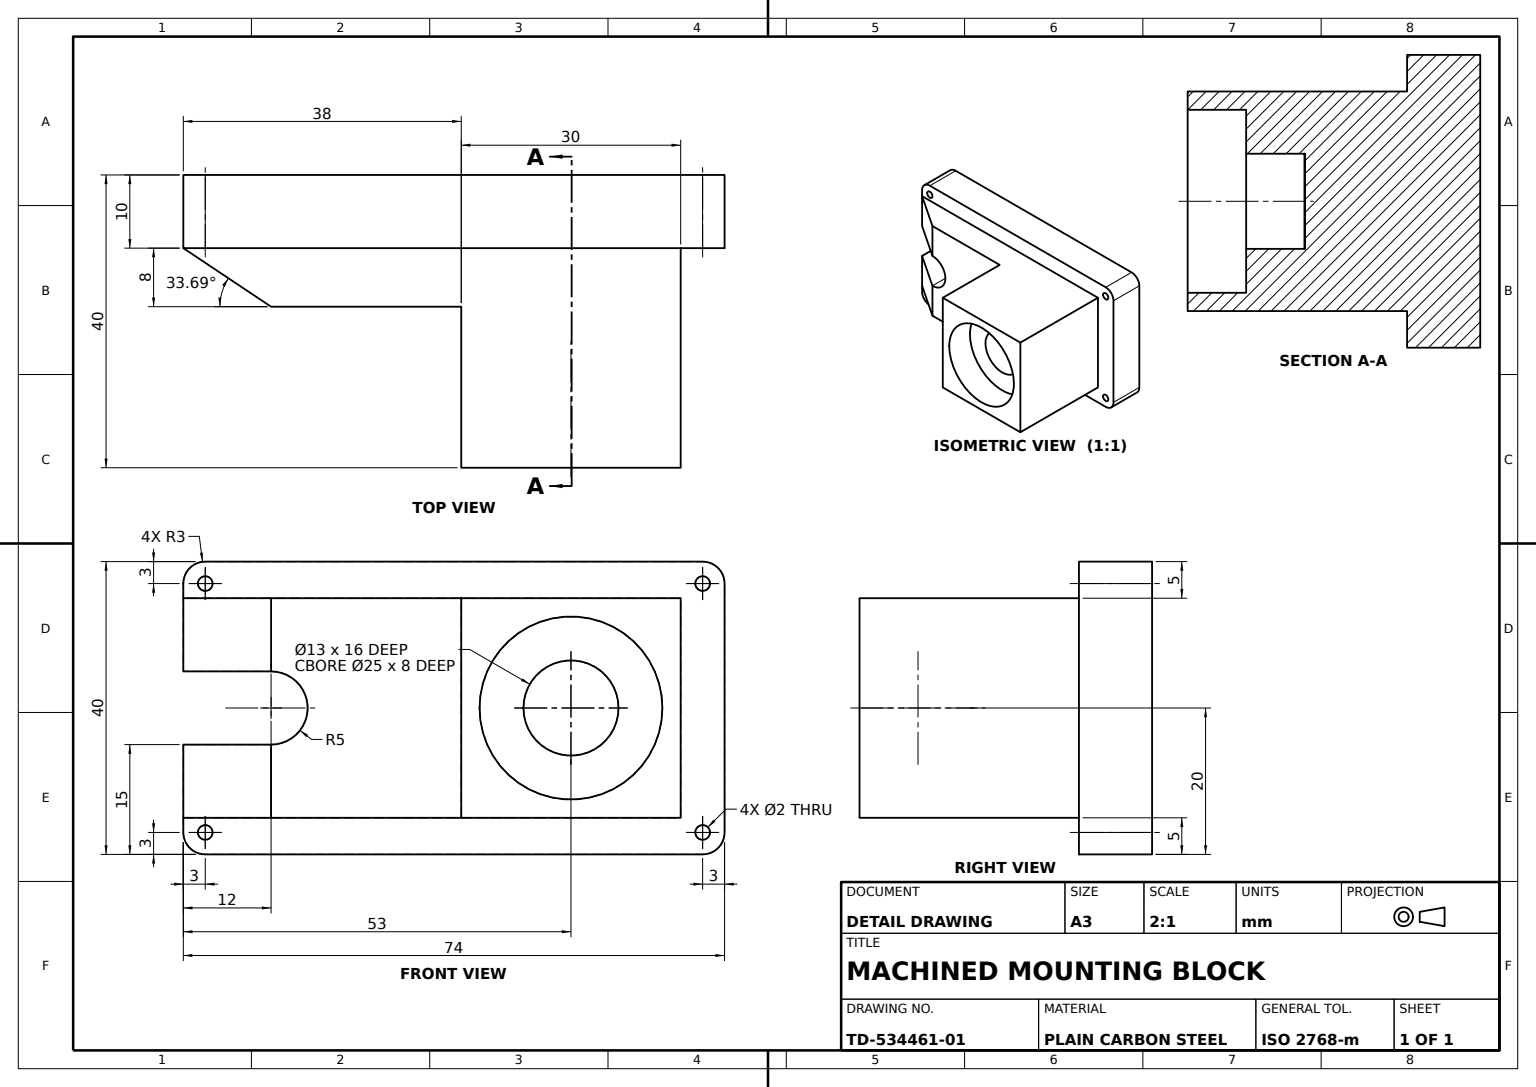
SolidWorks part; units mm, degrees
material "Plain Carbon Steel"
ref_plane "Front Plane" through (0, 0, 0) normal (0, 0, 1) x (1, 0, 0)
ref_plane "Top Plane" through (0, 0, 0) normal (0, 1, 0) x (1, 0, 0)
ref_plane "Right Plane" through (0, 0, 0) normal (1, 0, 0) x (0, 0, -1)
sketch "Flange Profile" plane through (0, 0, 0) normal (0, 0, 1) x (1, 0, 0)
  line L0 (3, 0) -> (71, 0)
  line L8 (74, 37) -> (74, 3)
  line L10 (3, 40) -> (71, 40)
  line L14 (12, 15) -> (0, 15)
  line L15 (12, 25) -> (0, 25)
  line L16 (0, 37) -> (0, 25)
  line L17 (0, 15) -> (0, 3)
  arc A0 (74, 37) -> (71, 40) centre (71, 37) ccw
  arc A1 (3, 40) -> (0, 37) centre (3, 37) ccw
  arc A2 (0, 3) -> (3, 0) centre (3, 3) ccw
  arc A3 (71, 0) -> (74, 3) centre (71, 3) ccw
  arc A4 (12, 15) -> (12, 25) centre (12, 20) ccw
  dimension "D1" = 6
  dimension "D2" = 6
  dimension "D3" = 6
  dimension "D4" = 6
  dimension "D5" = 10
  dimension "D6" = 3
  dimension "D9" = 5
  dimension "D7" = 74
  dimension "D8" = 40
  dimension "D10" = 12
  dimension "D11" = 20
extrude "Mounting Flange" add sketch "Flange Profile" along normal blind 10
sketch "Housing Block Profile" plane through (0, 0, 10) normal (0, 0, 1) x (1, 0, 0)
  line L0 (71, 40) -> (3, 40) construction
  line L1 (68, 35) -> (38, 35)
  line L2 (68, 35) -> (68, 5)
  line L3 (68, 5) -> (38, 5)
  line L4 (38, 35) -> (38, 5)
  line L5 (0, 37) -> (0, 25) construction
  line L9 (3, 0) -> (71, 0) construction
  point P4 (53, 5)
  dimension "D1" = 5
  dimension "D2" = 5
  dimension "D3" = 38
  dimension "D4" = 30
extrude "Housing Block" add sketch "Housing Block Profile" along normal blind 30
sketch "Upper Block Profile" plane through (38, 0, 0) normal (-1, 0, 0) x (0, 0, 1)
  line L0 (10, 35) -> (18, 35)
  line L1 (40, 35) -> (10, 35) construction
  line L2 (18, 35) -> (18, 5)
  line L3 (40, 5) -> (10, 5) construction
  line L4 (18, 5) -> (10, 5)
  line L5 (10, 5) -> (10, 35)
  line L6 (10, 35) -> (10, 5) construction
  dimension "D1" = 8
extrude "Upper Block" add sketch "Upper Block Profile" along normal blind 26
sketch "Side Relief Profile" plane through (0, 0, 10) normal (0, 0, -1) x (-1, 0, 0)
  line L0 (-12, 25) -> (-12, 15)
  arc A0 (-12, 25) -> (-12, 15) centre (-12, 20) ccw
  dimension "D1" = 10
extrude "Side Relief Cut" cut sketch "Side Relief Profile" against normal blind 8
sketch "Gusset A Profile" plane through (0, 5, 0) normal (0, -1, 0) x (1, 0, 0)
  line L0 (12, 10) -> (12, 18)
  line L1 (12, 18) -> (0, 10)
  line L2 (0, 10) -> (12, 10)
extrude "Gusset A" add sketch "Gusset A Profile" against normal blind 10
sketch "Gusset B Profile" plane through (0, 35, 0) normal (0, 1, 0) x (1, 0, 0)
  line L0 (12, -18) -> (12, -10)
  line L1 (12, -18) -> (0, -10) construction
  line L2 (12, -18) -> (12, -10) construction
  line L3 (12, -10) -> (0, -10)
  line L4 (0, -10) -> (12, -18)
extrude "Gusset B" add sketch "Gusset B Profile" against normal blind 10
sketch "Mounting Holes Profile" plane through (0, 0, 10) normal (0, 0, 1) x (1, 0, 0)
  line L0 (71, 40) -> (3, 40) construction
  line L1 (0, 37) -> (0, 35) construction
  line L2 (74, 3) -> (74, 37) construction
  line L3 (3, 0) -> (71, 0) construction
  circle A0 centre (3, 37) radius 1
  circle A1 centre (71, 37) radius 1
  circle A2 centre (71, 3) radius 1
  circle A3 centre (3, 3) radius 1
  dimension "D1" = 2
  dimension "D2" = 2
  dimension "D7" = 2
  dimension "D10" = 2
  dimension "D11" = 2
  dimension "D3" = 3
  dimension "D4" = 3
  dimension "D5" = 3
  dimension "D6" = 3
  dimension "D8" = 3
  dimension "D9" = 3
extrude "Mounting Holes 4x" cut sketch "Mounting Holes Profile" against normal blind 10
sketch "Counterbore Ø25 Profile" plane through (0, 0, 40) normal (0, 0, 1) x (1, 0, 0)
  line L0 (68, 5) -> (68, 35) construction
  line L1 (68, 35) -> (38, 35) construction
  circle A0 centre (53, 20) radius 12.5
  dimension "D1" = 25
  dimension "D2" = 25
  dimension "D3" = 15
  dimension "D4" = 15
extrude "Counterbore Ø25" cut sketch "Counterbore Ø25 Profile" against normal blind 8
sketch "Bore Ø13 Profile" plane through (0, 0, 32) normal (0, 0, 1) x (1, 0, 0)
  circle A0 centre (53, 20) radius 6.5
  dimension "D1" = 13
  dimension "D2" = 13
extrude "Bore Ø13" cut sketch "Bore Ø13 Profile" against normal blind 8
